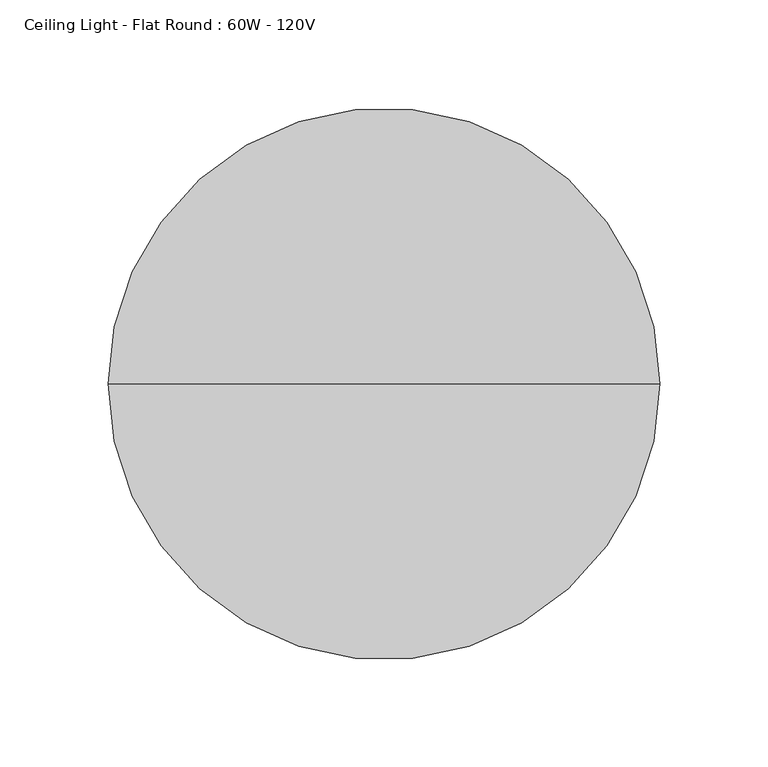
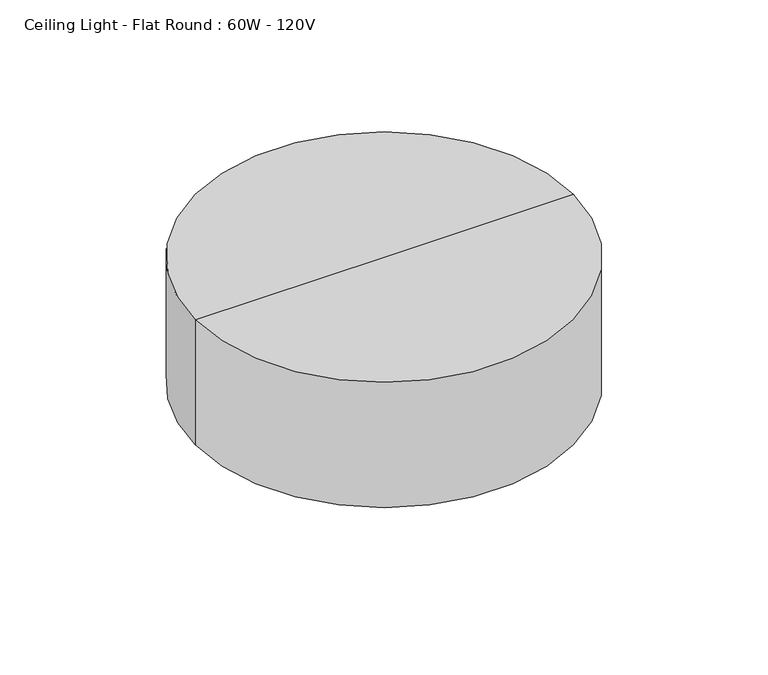
"""IFC4 building model written with IfcOpenShell, lengths in millimetres: light fixture geometry, Ceiling Light - Flat Round : 60W - 120V."""

from ifc_helpers import new_model, si_unit, point, frame, origin, origin_with_axes, origin_2d, place, context, project, spatial, polyline, circle_curve, trimmed, segment, composite_curve, outline, extrude, source, transform, mapped, element, save
from ifc_brep_helpers import plane_surface, cylinder_surface, revolved_surface, advanced_brep


def ceiling_light_flat_round_60w_120v_a3c1fe64(model_context):
    return source(origin(), model_context, "Body", "SolidModel", [
        extrude(outline(composite_curve([segment(trimmed(circle_curve(origin_2d(), 82.55), [point((-82.55, 0.0))], [point((82.55, 0.0))], False, "CARTESIAN"), True, "CONTINUOUS"), segment(trimmed(circle_curve(origin_2d(), 82.55), [point((82.55, 0.0))], [point((-82.55, 0.0))], False, "CARTESIAN"), True, "CONTINUOUS")], self_intersect=False), holes=[composite_curve([segment(trimmed(circle_curve(origin_2d(), 76.2), [point((-76.2, 0.0))], [point((76.2, 0.0))], True, "CARTESIAN"), True, "CONTINUOUS"), segment(trimmed(circle_curve(origin_2d(), 76.2), [point((76.2, 0.0))], [point((-76.2, 0.0))], True, "CARTESIAN"), True, "CONTINUOUS")], self_intersect=False)]), origin_with_axes(), (0.0, 0.0, 1.0), 25.4),
        advanced_brep(
        [(127.0, 0.0, 25.4), (-127.0, 0.0, 25.4), (-127.0, 0.0, 114.3), (127.0, 0.0, 114.3), (76.2, 0.0, 25.4), (-76.2, 0.0, 25.4), (76.2, 0.0, 0.0), (-76.2, 0.0, 0.0), (73.025, 0.0, 0.0), (-73.025, 0.0, 0.0), (73.025, 0.0, 28.575), (-73.025, 0.0, 28.575), (123.825, 0.0, 28.575), (-123.825, 0.0, 28.575), (123.825, 0.0, 111.125), (-123.825, 0.0, 111.125), (0.0, 0.0, 111.125), (0.0, 0.0, 114.3)],
        [
            (0, 1, circle_curve(frame((0.0, 0.0, 25.4), z_axis=(0.0, 0.0, 1.0), x_axis=(-1.0, 0.0, 0.0)), 127.0)),
            (1, 2),
            (2, 3, circle_curve(frame((0.0, 0.0, 114.3), z_axis=(0.0, 0.0, -1.0), x_axis=(-1.0, 0.0, 0.0)), 127.0)),
            (3, 0),
            (1, 0, circle_curve(frame((0.0, 0.0, 25.4), z_axis=(0.0, 0.0, 1.0), x_axis=(-1.0, 0.0, 0.0)), 127.0)),
            (3, 2, circle_curve(frame((0.0, 0.0, 114.3), z_axis=(0.0, 0.0, -1.0), x_axis=(-1.0, 0.0, 0.0)), 127.0)),
            (4, 5, circle_curve(frame((0.0, 0.0, 25.4), z_axis=(0.0, 0.0, 1.0), x_axis=(-1.0, 0.0, 0.0)), 76.2)),
            (5, 1),
            (0, 4),
            (5, 4, circle_curve(frame((0.0, 0.0, 25.4), z_axis=(0.0, 0.0, 1.0), x_axis=(-1.0, 0.0, 0.0)), 76.2)),
            (6, 7, circle_curve(frame((0.0, 0.0, 0.0), z_axis=(0.0, 0.0, 1.0), x_axis=(-1.0, 0.0, 0.0)), 76.2)),
            (7, 5),
            (4, 6),
            (7, 6, circle_curve(frame((0.0, 0.0, 0.0), z_axis=(0.0, 0.0, 1.0), x_axis=(-1.0, 0.0, 0.0)), 76.2)),
            (8, 9, circle_curve(frame((0.0, 0.0, 0.0), z_axis=(0.0, 0.0, 1.0), x_axis=(-1.0, 0.0, 0.0)), 73.025)),
            (9, 7),
            (6, 8),
            (9, 8, circle_curve(frame((0.0, 0.0, 0.0), z_axis=(0.0, 0.0, 1.0), x_axis=(-1.0, 0.0, 0.0)), 73.025)),
            (10, 11, circle_curve(frame((0.0, 0.0, 28.575), z_axis=(0.0, 0.0, 1.0), x_axis=(-1.0, 0.0, 0.0)), 73.025)),
            (11, 9),
            (8, 10),
            (11, 10, circle_curve(frame((0.0, 0.0, 28.575), z_axis=(0.0, 0.0, 1.0), x_axis=(-1.0, 0.0, 0.0)), 73.025)),
            (12, 13, circle_curve(frame((0.0, 0.0, 28.575), z_axis=(0.0, 0.0, 1.0), x_axis=(-1.0, 0.0, 0.0)), 123.825)),
            (13, 11),
            (10, 12),
            (13, 12, circle_curve(frame((0.0, 0.0, 28.575), z_axis=(0.0, 0.0, 1.0), x_axis=(-1.0, 0.0, 0.0)), 123.825)),
            (14, 15, circle_curve(frame((0.0, 0.0, 111.125), z_axis=(0.0, 0.0, 1.0), x_axis=(-1.0, 0.0, 0.0)), 123.825)),
            (15, 13),
            (12, 14),
            (15, 14, circle_curve(frame((0.0, 0.0, 111.125), z_axis=(0.0, 0.0, 1.0), x_axis=(-1.0, 0.0, 0.0)), 123.825)),
            (16, 15),
            (14, 16),
            (2, 17),
            (17, 3),
        ],
        [
            cylinder_surface(frame((0.0, 0.0, 111.125), z_axis=(0.0, 0.0, -1.0), x_axis=(-1.0, 0.0, 0.0)), 127.0),
            plane_surface(frame((0.0, 0.0, 25.4), z_axis=(0.0, 0.0, -1.0), x_axis=(-1.0, 0.0, 0.0))),
            cylinder_surface(frame((0.0, 0.0, 111.125), z_axis=(0.0, 0.0, -1.0), x_axis=(-1.0, 0.0, 0.0)), 76.2),
            plane_surface(frame((0.0, 0.0, 0.0), z_axis=(0.0, 0.0, -1.0), x_axis=(-1.0, 0.0, 0.0))),
            revolved_surface(polyline([(-73.025, 0.0, 0.0), (-73.025, 0.0, 28.575000000000003)]), (0.0, 0.0, 111.125), (0.0, 0.0, -1.0)),
            plane_surface(frame((0.0, 0.0, 28.575), z_axis=(0.0, 0.0, 1.0), x_axis=(-1.0, 0.0, 0.0))),
            revolved_surface(polyline([(-123.825, 0.0, 28.575000000000003), (-123.825, 0.0, 111.125)]), (0.0, 0.0, 111.125), (0.0, 0.0, -1.0)),
            plane_surface(frame((0.0, 0.0, 111.125), z_axis=(0.0, 0.0, -1.0), x_axis=(-1.0, 0.0, 0.0))),
            plane_surface(frame((0.0, 0.0, 114.3), z_axis=(0.0, 0.0, 1.0), x_axis=(-1.0, 0.0, 0.0))),
        ],
        [
            (0, [[1, 2, 3, 4]]),
            (0, [[5, -4, 6, -2]]),
            (1, [[7, 8, -1, 9]]),
            (1, [[10, -9, -5, -8]]),
            (2, [[11, 12, -7, 13]]),
            (2, [[14, -13, -10, -12]]),
            (3, [[15, 16, -11, 17]]),
            (3, [[18, -17, -14, -16]]),
            (4, [[19, 20, -15, 21]]),
            (4, [[22, -21, -18, -20]]),
            (5, [[23, 24, -19, 25]]),
            (5, [[26, -25, -22, -24]]),
            (6, [[27, 28, -23, 29]]),
            (6, [[30, -29, -26, -28]]),
            (7, [[31, -27, 32]]),
            (7, [[-32, -30, -31]]),
            (8, [[-3, 33, 34]]),
            (8, [[-6, -34, -33]]),
        ],
    ),
    ])


if __name__ == "__main__":
    model = new_model("IFC4")
    model_context = context("Model", 3, world=origin())
    ifc_project = project(units=[si_unit("LENGTHUNIT", "METRE", prefix="MILLI")], contexts=[model_context])
    site = spatial("IfcSite", under=ifc_project)
    building = spatial("IfcBuilding", under=site)
    placement = place(None, origin())
    ceiling_light_flat_round_60w_120v_shape = ceiling_light_flat_round_60w_120v_a3c1fe64(model_context)
    element("IfcLightFixture", 1, ObjectType="Ceiling Light - Flat Round : 60W - 120V", at=placement, inside=building, context=model_context, shape_type="MappedRepresentation", body=[
        mapped(ceiling_light_flat_round_60w_120v_shape, transform((0.0, 0.0, 0.0), x_axis=(1.0, 0.0, 0.0), y_axis=(0.0, 1.0, 0.0), z_axis=(0.0, 0.0, 1.0))),
    ])
    save(model, "model.ifc")

# Revit data of these elements
# Type "Ceiling Light - Flat Round : 60W - 120V"
#   Lamp = "A-19"
#   Photometric Web File = "CLFR1A19.ies"
#   Assembly Code = "D5020220"
#   Wattage = 60 W
#   built-in parameter 1150110 = 1 (stored number, unit not read)
#   built-in parameter 1150109 = 1 (stored number, unit not read)
#   built-in parameter 1150113 = 1 (stored number, unit not read)
#   Tilt Angle = -90.00°
#   built-in parameter 1150115 = 1 (stored number, unit not read)
#   built-in parameter 1150105 = 68.0387 (stored number, unit not read)
#   built-in parameter 1150112 = 1 (stored number, unit not read)
#   built-in parameter 1150114 = 1 (stored number, unit not read)
#   built-in parameter 1150107 = 2800 (stored number, unit not read)
#   built-in parameter 1150106 = 0.680387 (stored number, unit not read)
#   Emit from Circle Diameter = 0' - 10"
#   built-in parameter 1150104 = 1.32387 (stored number, unit not read)
#   Lumens = 855 lm
#   built-in parameter 1114217 = 1 (stored number, unit not read)
#   Default Elevation = 4' - 0"
#   Ballast Voltage = 120 V
#   built-in parameter 1114218 = 1 (stored number, unit not read)
#   built-in parameter 1150133 = 10 (stored number, unit not read)
#   Apparent Load = 60 VA
#   built-in parameter 1150134 = 4
#   built-in parameter 1150137 = 1
#   Color Filter = 16777215
#   built-in parameter 1140040 [instance default] = 1
#   Ballast Number of Poles = 1
#   Light Box Material = Steel, Paint Finish, Dark Gray, Matte
#   Diffuser Material = Glass, White, High Luminance
#   Emit Shape Visible in Rendering = no
#   Dimming Lamp Color Temperature Shift = (empty or 0)
# Element 1 (IfcLightFixture, "Ceiling Light - Flat Round : 60W - 120V")
#   Materials on its faces: "Glass, White, High Luminance", "Steel, Paint Finish, Dark Gray, Matte"
# Materials
#   "Steel, Paint Finish, Dark Gray, Matte": class "Metal", colour RGB 98 98 98, transparency 0, Description = "Steel, paint finish, dark gray, matte", Cost = 0
#   "Glass, White, High Luminance": class "Glass", colour RGB 249 250 249, transparency 0.8, Description = "physical material", Cost = 0
